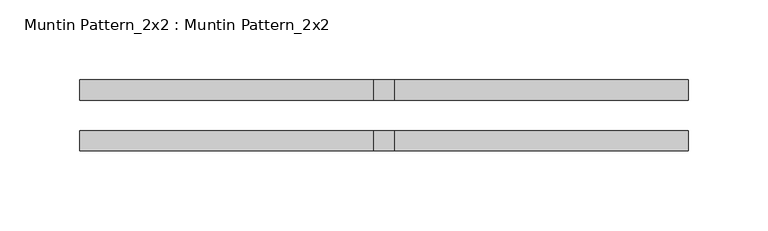
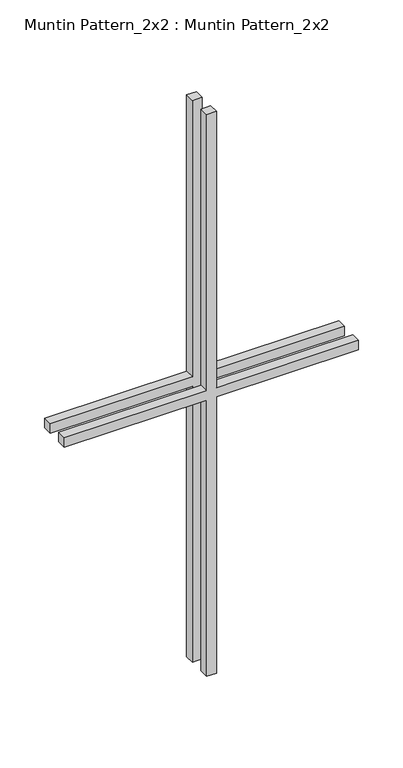
"""IFC4 building model written with IfcOpenShell, lengths in millimetres: proxy geometry, Muntin Pattern_2x2 : Muntin Pattern_2x2."""

from ifc_helpers import new_model, si_unit, frame, origin, place, context, project, spatial, polyline, outline, extrude, source, transform, mapped, element, save


def muntin_pattern_2x2_muntin_pattern_2x2_31a16349(model_context):
    return source(origin(), model_context, "Body", "SweptSolid", [
        extrude(outline(polyline([(390.525, -6.35), (390.525, -190.5), (377.825, -190.5), (377.825, -6.35), (0.0, -6.35), (0.0, 6.35), (377.825, 6.35), (377.825, 190.5), (390.525, 190.5), (390.525, 6.35), (768.35, 6.35), (768.35, -6.35), (390.525, -6.35)])), frame((0.0, 9.525, 0.0), z_axis=(0.0, 1.0, 0.0), x_axis=(0.0, 0.0, 1.0)), (0.0, 0.0, 1.0), 12.7),
        extrude(outline(polyline([(390.525, -6.35), (390.525, -190.5), (377.825, -190.5), (377.825, -6.35), (0.0, -6.35), (0.0, 6.35), (377.825, 6.35), (377.825, 190.5), (390.525, 190.5), (390.525, 6.35), (768.35, 6.35), (768.35, -6.35), (390.525, -6.35)])), frame((0.0, -22.225, 0.0), z_axis=(0.0, 1.0, 0.0), x_axis=(0.0, 0.0, 1.0)), (0.0, 0.0, 1.0), 12.7),
    ])


if __name__ == "__main__":
    model = new_model("IFC4")
    model_context = context("Model", 3, world=origin())
    ifc_project = project(units=[si_unit("LENGTHUNIT", "METRE", prefix="MILLI")], contexts=[model_context])
    site = spatial("IfcSite", under=ifc_project)
    building = spatial("IfcBuilding", under=site)
    placement = place(None, origin())
    muntin_pattern_2x2_muntin_pattern_2x2_shape = muntin_pattern_2x2_muntin_pattern_2x2_31a16349(model_context)
    element("IfcBuildingElementProxy", 1, Name="Muntin Pattern_2x2 : Muntin Pattern_2x2", ObjectType="Muntin Pattern_2x2 : Muntin Pattern_2x2", at=placement, inside=building, context=model_context, shape_type="MappedRepresentation", body=[
        mapped(muntin_pattern_2x2_muntin_pattern_2x2_shape, transform((0.0, 0.0, 0.0), x_axis=(1.0, 0.0, 0.0), y_axis=(0.0, 1.0, 0.0), z_axis=(0.0, 0.0, 1.0))),
    ])
    save(model, "model.ifc")

# Revit data of these elements
# Type "Muntin Pattern_2x2 : Muntin Pattern_2x2"
#   Width [instance default] = 4' - 0"
#   Thickness = 0' - 0 1/2"
#   Height [instance default] = 4' - 0"
#   Distance = 0' - 0 3/4"
#   Interior Material [instance default] = none
#   Exterior Material [instance default] = none
#   Default Elevation = 0
# Element 1 (IfcBuildingElementProxy, "Muntin Pattern_2x2 : Muntin Pattern_2x2")
#   Width = 1' - 3"
#   Height = 2' - 6 1/4"
#   Interior Material = Wood - Stained
#   Exterior Material = Clad - White
#   Materials on its faces: "Clad - White", "Wood - Stained"
# Materials
#   "Clad - White": class "Wood", colour RGB 242 242 238, transparency 0, Cost = 0
#   "Wood - Stained": class "Wood", colour RGB 224 178 126, transparency 0, Cost = 0
